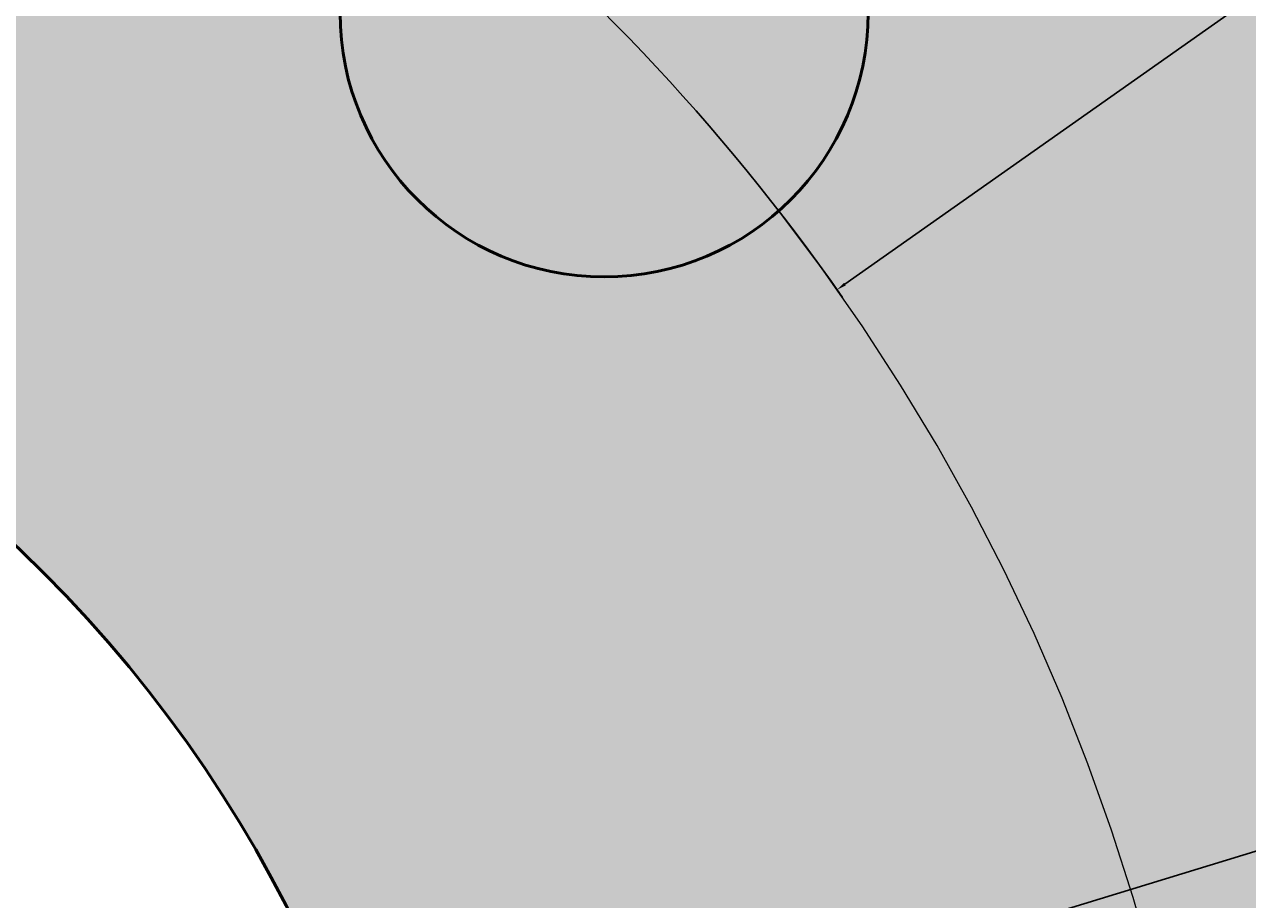
# Model space of a CAD drawing. Units: inches. Extents: x 139261 to 139415, y 52839 to 52963.
# Tile 16 of 20: x 139358 to 139381, y 52912 to 52928. Entities that reach past the tile are written whole.
import ezdxf

# ---------------------------------------------------------------- set-up
doc = ezdxf.new("R2010")
doc.units = ezdxf.units.IN
doc.header["$MEASUREMENT"] = 0
doc.linetypes.add('CENTER', pattern=[50.8, 31.75, -6.35, 6.35, -6.35])
for name, color, linetype, lineweight in [('M-CNTR', 4, 'CENTER', 18), ('M-DIMS', 2, 'Continuous', 25), ('M-HATC', 8, 'Continuous', 18), ('M-OUTL', 7, 'Continuous', 50)]:
    doc.layers.add(name, color=color, linetype=linetype, lineweight=lineweight)
doc.styles.get("Standard").update_dxf_attribs({"font": 'arial.ttf'})
doc.dimstyles.get("Standard").update_dxf_attribs({"dimtxt": 0.18, "dimasz": 0.18, "dimexe": 0.18, "dimexo": 0.0625, "dimgap": 0.09, "dimtad": 0, "dimtih": 1, "dimtoh": 1, "dimdec": 4, "dimzin": 0, "dimdsep": 46, "dimtxsty": 'Standard', "dimcen": 0.09, "dimadec": 0, "dimazin": 0, "dimtfac": 1, "dimtdec": 4, "dimtofl": 0, "dimtmove": 0, "dimatfit": 3, "dimfxl": 1, "dimtolj": 1, "dimtzin": 0, "dimarcsym": 0})

# ---------------------------------------------------------------- blocks, each defined once
blk = doc.blocks.new('*U1')
blk.add_circle((0, 0), 5)
blk = doc.blocks.new('*U2')
at = {"layer": 'M-OUTL', "color": 0, "linetype": 'ByBlock', "lineweight": -2, "transparency": 16777216, "rotation": 315}
blk.add_blockref('*U1', (139368.641, 52928.502), dxfattribs=at)
blk = doc.blocks.new('*D3')
at = {"layer": 'Defpoints', "color": 0, "transparency": 16777216}
for p in [(139359.484, 52906.062), (139321.23, 52894.373)]:
    blk.add_point(p, dxfattribs=at)
at = {"layer": 'M-DIMS', "color": 0, "lineweight": -2, "transparency": 16777216}
for p, q in [((139412.091, 52922.136), (139359.656, 52906.115)), ((139412.271, 52922.136), (139412.091, 52922.136)), ((139340.357, 52900.127), (139340.357, 52900.307)), ((139340.267, 52900.217), (139340.447, 52900.217))]:
    blk.add_line(p, q, dxfattribs=at)
at = {"layer": 'M-DIMS', "color": 0, "transparency": 16777216}
blk.add_solid([(139359.647, 52906.143), (139359.665, 52906.086), (139359.484, 52906.062)], dxfattribs=at)
at = {"layer": 'M-DIMS', "color": 0, "transparency": 16777216, "insert": (139412.902, 52922.136), "char_height": 0.18, "attachment_point": 5}
blk.add_mtext('\\A1;∅40.0000', dxfattribs=at)
blk = doc.blocks.new('*D4')
at = {"layer": 'Defpoints', "color": 0, "transparency": 16777216}
for p in [(139373.053, 52923.26), (139307.661, 52877.175)]:
    blk.add_point(p, dxfattribs=at)
at = {"layer": 'M-DIMS', "color": 0, "lineweight": -2, "transparency": 16777216}
for p, q in [((139414.011, 52952.126), (139373.2, 52923.364)), ((139414.191, 52952.126), (139414.011, 52952.126)), ((139340.357, 52900.127), (139340.357, 52900.307)), ((139340.267, 52900.217), (139340.447, 52900.217))]:
    blk.add_line(p, q, dxfattribs=at)
blk.add_arc((139340.357, 52900.217), 40, 34.9168, 52.0771, dxfattribs=at)
at = {"layer": 'M-DIMS', "color": 0, "transparency": 16777216}
blk.add_solid([(139373.183, 52923.388), (139373.217, 52923.339), (139373.053, 52923.26)], dxfattribs=at)
at = {"layer": 'M-DIMS', "color": 0, "transparency": 16777216, "insert": (139414.822, 52952.126), "char_height": 0.18, "attachment_point": 5}
blk.add_mtext('\\A1;∅80.0000', dxfattribs=at)
blk = doc.blocks.new('*D5')
at = {"layer": 'Defpoints', "color": 0, "transparency": 16777216}
for p in [(139316.763, 52908.484), (139363.951, 52891.951)]:
    blk.add_point(p, dxfattribs=at)
at = {"layer": 'M-DIMS', "color": 0, "lineweight": -2, "transparency": 16777216}
for p, q in [((139262.553, 52927.414), (139262.733, 52927.414)), ((139262.733, 52927.414), (139316.593, 52908.544)), ((139340.357, 52900.127), (139340.357, 52900.307)), ((139340.267, 52900.217), (139340.447, 52900.217))]:
    blk.add_line(p, q, dxfattribs=at)
at = {"layer": 'M-DIMS', "color": 0, "transparency": 16777216}
blk.add_solid([(139316.603, 52908.572), (139316.583, 52908.515), (139316.763, 52908.484)], dxfattribs=at)
at = {"layer": 'M-DIMS', "color": 0, "transparency": 16777216, "insert": (139261.922, 52927.414), "char_height": 0.18, "attachment_point": 5}
blk.add_mtext('\\A1;∅50.0000', dxfattribs=at)
blk = doc.blocks.new('*D9')
at = {"layer": 'Defpoints', "color": 0, "transparency": 16777216}
for p in [(139302.054, 52932.357), (139378.659, 52868.078)]:
    blk.add_point(p, dxfattribs=at)
at = {"layer": 'M-DIMS', "color": 0, "lineweight": -2, "transparency": 16777216}
for p, q in [((139278.893, 52951.64), (139279.073, 52951.64)), ((139279.073, 52951.64), (139301.916, 52932.472)), ((139340.357, 52900.127), (139340.357, 52900.307)), ((139340.267, 52900.217), (139340.447, 52900.217))]:
    blk.add_line(p, q, dxfattribs=at)
at = {"layer": 'M-DIMS', "color": 0, "transparency": 16777216}
blk.add_solid([(139301.936, 52932.495), (139301.897, 52932.449), (139302.054, 52932.357)], dxfattribs=at)
at = {"layer": 'M-DIMS', "color": 0, "transparency": 16777216, "insert": (139278.506, 52951.64), "char_height": 0.18, "attachment_point": 5}
blk.add_mtext('\\A1;∅100', dxfattribs=at)
blk = doc.blocks.new('*D10')
at = {"layer": 'Defpoints', "color": 0, "transparency": 16777216}
for p in [(139325.07, 52937.181), (139355.644, 52863.254)]:
    blk.add_point(p, dxfattribs=at)
at = {"layer": 'M-DIMS', "color": 0, "lineweight": -2, "transparency": 16777216}
for p, q in [((139340.357, 52900.127), (139340.357, 52900.307)), ((139340.267, 52900.217), (139340.447, 52900.217)), ((139364.816, 52841.075), (139355.712, 52863.087)), ((139364.996, 52841.075), (139364.816, 52841.075))]:
    blk.add_line(p, q, dxfattribs=at)
at = {"layer": 'M-DIMS', "color": 0, "transparency": 16777216}
blk.add_solid([(139355.74, 52863.099), (139355.685, 52863.076), (139355.644, 52863.254)], dxfattribs=at)
at = {"layer": 'M-DIMS', "color": 0, "transparency": 16777216, "insert": (139365.312, 52841.075), "char_height": 0.18, "attachment_point": 5}
blk.add_mtext('\\A1;∅80', dxfattribs=at)

msp = doc.modelspace()

# ---------------------------------------------------------------- hatches: boundary and pattern name
at = {"layer": 'M-HATC'}
h = msp.add_hatch(color=256, dxfattribs=at)
h.dxf.hatch_style = 1
h.paths.add_polyline_path([(139290.35689, 52900.21749, 1), (139390.35689, 52900.21749, 1)])
h.paths.add_polyline_path([(139335.36666, 52939.90499, -0.01563646), (139335.35689, 52940.21749, -1), (139345.35689, 52940.21749, -0.01563646), (139345.34711, 52939.90499, -0.13461315), (139364.89157, 52931.80941, -0.691035), (139373.64116, 52928.50176, -0.21521822), (139371.94881, 52924.75216, -0.13461315), (139380.04439, 52905.20771, -0.43265224), (139385.35689, 52900.21749, -0.43265224), (139380.04439, 52895.22726, -0.13461315), (139371.94881, 52875.68281, -0.21521822), (139373.64116, 52871.93321, -0.691035), (139364.89157, 52868.62556, -0.13461315), (139345.34711, 52860.52999, -0.01563646), (139345.35689, 52860.21749, -1), (139335.35689, 52860.21749, -0.01563646), (139335.36666, 52860.52999, -0.13461315), (139315.82221, 52868.62556, -0.691035), (139307.07262, 52871.93321, -0.21521822), (139308.76496, 52875.68281, -0.13461315), (139300.66939, 52895.22726, -0.43265224), (139295.35689, 52900.21749, -0.43265224), (139300.66939, 52905.20771, -0.13461315), (139308.76496, 52924.75216, -0.21521822), (139307.07262, 52928.50176, -0.691035), (139315.82221, 52931.80941, -0.13461315)], flags=16)
h.paths.add_polyline_path([(139365.35689, 52900.21749, -1), (139315.35689, 52900.21749, -1)], flags=0)
h.paths.add_polyline_path([(139323.71474, 52911.30978), (139356.99903, 52911.30978, -0.3027197), (139356.99903, 52889.12519), (139323.71474, 52889.12519, -0.3027197)], flags=0)
h.paths.add_polyline_path([(139364.89157, 52931.80941, 0.13461315), (139345.34711, 52939.90499, -0.93933644), (139335.36666, 52939.90499, 0.13461315), (139315.82221, 52931.80941, -0.18270763), (139317.07262, 52928.50176, -0.64579494), (139308.76496, 52924.75216, 0.13461315), (139300.66939, 52905.20771, -0.39601219), (139305.35689, 52900.21749, -0.39601219), (139300.66939, 52895.22726, 0.13461315), (139308.76496, 52875.68281, -0.64579494), (139317.07262, 52871.93321, -0.18270763), (139315.82221, 52868.62556, 0.13461315), (139335.36666, 52860.52999, -0.93933644), (139345.34711, 52860.52999, 0.13461315), (139364.89157, 52868.62556, -0.18270763), (139363.64116, 52871.93321, -0.64579494), (139371.94881, 52875.68281, 0.13461315), (139380.04439, 52895.22726, -0.39601219), (139375.35689, 52900.21749, -0.39601219), (139380.04439, 52905.20771, 0.13461315), (139371.94881, 52924.75216, -0.64579494), (139363.64116, 52928.50176, -0.18270763)], flags=0)
h = msp.add_hatch(color=256, dxfattribs=at)
h.dxf.hatch_style = 1
h.set_gradient(color1=(205, 105, 40), tint=1)
h.paths.add_polyline_path([(139335.35689, 52940.21749, 1), (139345.35689, 52940.21749, 1)])
h.paths.add_polyline_path([(139307.07262, 52928.50176, 1), (139317.07262, 52928.50176, 1)])
h.paths.add_polyline_path([(139295.35689, 52900.21749, 1), (139305.35689, 52900.21749, 1)])
h.paths.add_polyline_path([(139307.07262, 52871.93321, 1), (139317.07262, 52871.93321, 1)])
h.paths.add_polyline_path([(139345.35689, 52860.21749, 1), (139335.35689, 52860.21749, 1)])
h.paths.add_polyline_path([(139363.64116, 52871.93321, 1), (139373.64116, 52871.93321, 1)])
h.paths.add_polyline_path([(139375.35689, 52900.21749, 1), (139385.35689, 52900.21749, 1)])
h.paths.add_polyline_path([(139363.64116, 52928.50176, 1), (139373.64116, 52928.50176, 1)])
h = msp.add_hatch(color=256, dxfattribs=at)
h.dxf.hatch_style = 1
h.paths.add_polyline_path([(139345.34711, 52939.90499, -0.93933644), (139335.36666, 52939.90499, 0.13461315), (139315.82221, 52931.80941, -0.18270763), (139317.07262, 52928.50176, -0.64579494), (139308.76496, 52924.75216, 0.13461315), (139300.66939, 52905.20771, -0.39601219), (139305.35689, 52900.21749, -0.39601219), (139300.66939, 52895.22726, 0.13461315), (139308.76496, 52875.68281, -0.64579494), (139317.07262, 52871.93321, -0.18270763), (139315.82221, 52868.62556, 0.13461315), (139335.36666, 52860.52999, -0.93933644), (139345.34711, 52860.52999, 0.13461315), (139364.89157, 52868.62556, -0.18270763), (139363.64116, 52871.93321, -0.64579494), (139371.94881, 52875.68281, 0.13461315), (139380.04439, 52895.22726, -0.39601219), (139375.35689, 52900.21749, -0.39601219), (139380.04439, 52905.20771, 0.13461315), (139371.94881, 52924.75216, -0.64579494), (139363.64116, 52928.50176, -0.18270763), (139364.89157, 52931.80941, 0.13461315)])
h.paths.add_polyline_path([(139365.35689, 52900.21749, -1), (139315.35689, 52900.21749, -1)], flags=16)
h.paths.add_polyline_path([(139356.99903, 52911.30978, -0.3027197), (139356.99903, 52889.12519), (139323.71474, 52889.12519, -0.3027197), (139323.71474, 52911.30978)], flags=0)

# ---------------------------------------------------------------- linework, layer by layer
at = {"layer": 'M-CNTR'}
msp.add_arc((139340.35689, 52900.21749), 40, 7.166643, 37.833357, dxfattribs=at)
at = {"layer": 'M-OUTL'}
for radius in [50, 25]:
    msp.add_circle((139340.35689, 52900.21749), radius, dxfattribs=at)

# ---------------------------------------------------------------- block references
msp.add_blockref('*U2', (0, 0), dxfattribs=at)

# ---------------------------------------------------------------- dimensions: what is measured, and where the dimension line sits
at = {"layer": 'M-DIMS'}
for p1, p2, override, picture, middle in [((139307.66087, 52877.17469), (139373.0529, 52923.26028), {"dimclrd": 0, "dimclre": 0, "dimclrt": 0}, '*D4', (139414.82217, 52952.12585)), ((139378.65939, 52868.07845), (139302.05438, 52932.35652), {"dimdec": 0, "dimlfac": 1, "dimrnd": 0, "dimzin": 0, "dimdsep": 46, "dimlunit": 2}, '*D9', (139278.50641, 52951.63995)), ((139325.07023, 52937.18123), (139355.64354, 52863.25374), {"dimdec": 0, "dimlfac": 1, "dimrnd": 0, "dimzin": 0, "dimdsep": 46, "dimlunit": 2}, '*D10', (139365.31206, 52841.0755)), ((139363.95063, 52891.95098), (139316.76314, 52908.48399), {"dimclrd": 0, "dimclre": 0, "dimclrt": 0}, '*D5', (139261.92224, 52927.41429)), ((139321.22987, 52894.37307), (139359.4839, 52906.0619), {"dimclrd": 0, "dimclre": 0, "dimclrt": 0}, '*D3', (139412.90184, 52922.13633))]:
    dim = msp.add_diameter_dim_2p(p1=p1, p2=p2, dimstyle='Standard', override=override, dxfattribs=at)
    dim.commit()
    dim.dimension.update_dxf_attribs({"geometry": picture, "text_midpoint": middle, "dimtype": 163})

doc.saveas('drawing.dxf')
